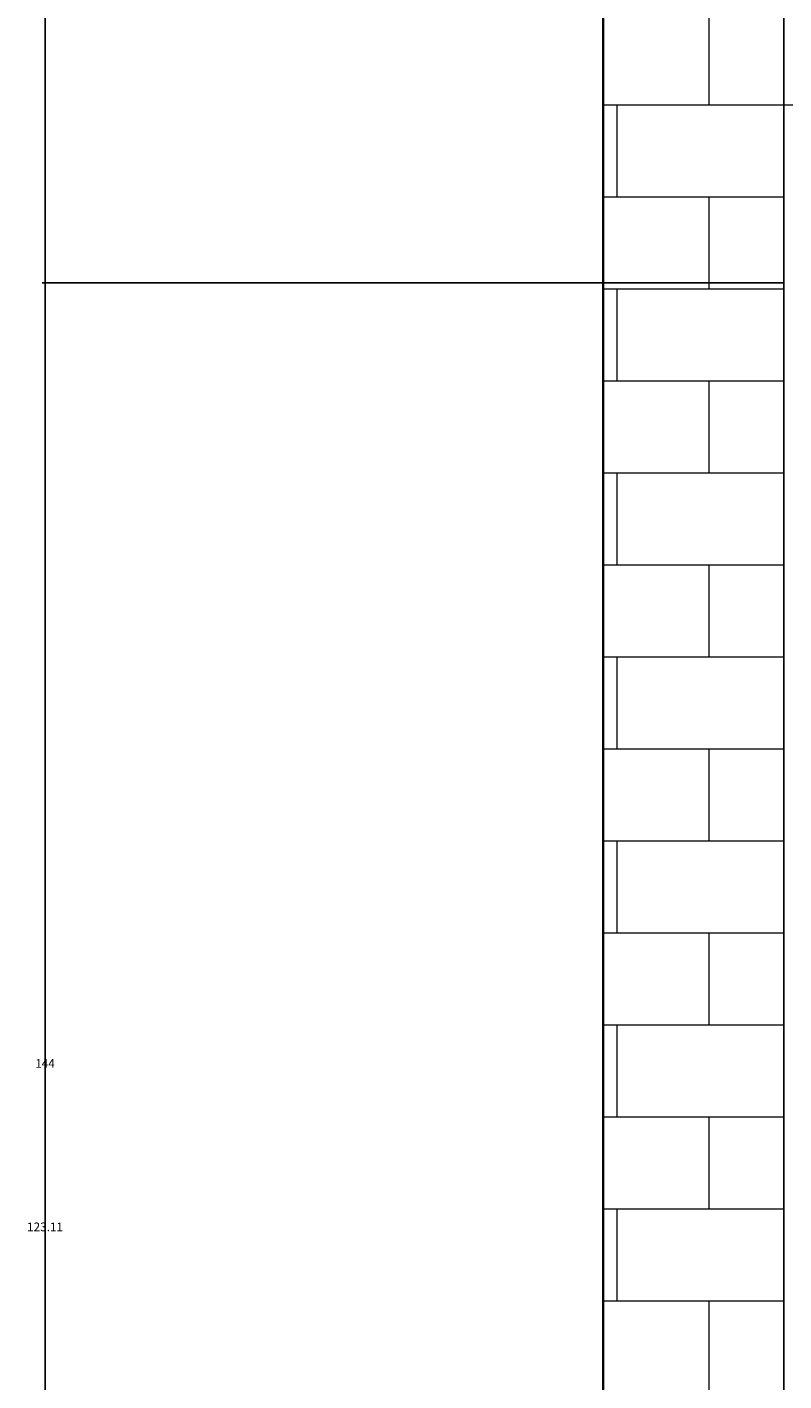
# Model space of a CAD drawing. Units: inches. Extents: x -26 to 776, y -22 to 650.
# Tile 3 of 62: x -26 to 23, y 67 to 155. Entities that reach past the tile are written whole.
import ezdxf

# ---------------------------------------------------------------- set-up
doc = ezdxf.new("R2010")
doc.units = ezdxf.units.IN
doc.header["$MEASUREMENT"] = 0
for name, color, linetype, lineweight in [('A-ANNO-DIMS', 2, 'Continuous', 18), ('A-WALL', 7, 'Continuous', 35), ('A-WALL-PATT', 8, 'Continuous', 13)]:
    doc.layers.add(name, color=color, linetype=linetype, lineweight=lineweight)
doc.styles.get("Standard").update_dxf_attribs({"font": 'arial.ttf'})
doc.dimstyles.get("Standard").update_dxf_attribs({"dimtxt": 0.5625, "dimasz": 0.18, "dimexe": 0.18, "dimexo": 0.0625, "dimgap": 0.09, "dimtad": 0, "dimtih": 1, "dimtoh": 1, "dimdec": 4, "dimzin": 0, "dimdsep": 46, "dimlunit": 4, "dimtxsty": 'Standard', "dimcen": 0.09, "dimadec": 0, "dimazin": 0, "dimtfac": 1, "dimtdec": 4, "dimtofl": 0, "dimtmove": 0, "dimatfit": 3, "dimfxl": 1, "dimtolj": 1, "dimtzin": 0, "dimarcsym": 0})

# ---------------------------------------------------------------- blocks, each defined once
blk = doc.blocks.new('*D14')
at = {"layer": 'A-ANNO-DIMS', "color": 0, "lineweight": -2, "transparency": 16777216}
for p, q in [((191.616, 613.271), (-25.478, 613.271)), ((-25.298, 613.091), (-25.298, 314.754)), ((-25.298, 15.662), (-25.298, 314)), ((11.045, 15.482), (-25.478, 15.482))]:
    blk.add_line(p, q, dxfattribs=at)
at = {"layer": 'A-ANNO-DIMS', "color": 0, "transparency": 16777216}
for points in [[(-25.328, 613.091), (-25.268, 613.091), (-25.298, 613.271)], [(-25.328, 15.662), (-25.268, 15.662), (-25.298, 15.482)]]:
    blk.add_solid(points, dxfattribs=at)
at = {"layer": 'Defpoints', "color": 0, "transparency": 16777216}
for p in [(-25.298, 613.271), (191.678, 613.271), (11.107, 15.482)]:
    blk.add_point(p, dxfattribs=at)
at = {"layer": 'A-ANNO-DIMS', "color": 0, "transparency": 16777216, "insert": (-25.298, 314.377), "char_height": 0.5625, "attachment_point": 5}
blk.add_mtext('\\A1;597.8', dxfattribs=at)
blk = doc.blocks.new('*D22')
at = {"layer": 'A-ANNO-DIMS', "color": 0, "lineweight": -2, "transparency": 16777216}
for p, q in [((22.889, 15.333), (22.889, 649.856)), ((217.953, 15.545), (217.953, 649.856)), ((23.069, 649.676), (119.19, 649.676)), ((217.773, 649.676), (121.652, 649.676))]:
    blk.add_line(p, q, dxfattribs=at)
at = {"layer": 'A-ANNO-DIMS', "color": 0, "transparency": 16777216}
for points in [[(23.069, 649.706), (23.069, 649.646), (22.889, 649.676)], [(217.773, 649.706), (217.773, 649.646), (217.953, 649.676)]]:
    blk.add_solid(points, dxfattribs=at)
at = {"layer": 'Defpoints', "color": 0, "transparency": 16777216}
for p in [(217.953, 649.676), (22.889, 15.27), (217.953, 15.482)]:
    blk.add_point(p, dxfattribs=at)
at = {"layer": 'A-ANNO-DIMS', "color": 0, "transparency": 16777216, "insert": (120.421, 649.676), "char_height": 0.5625, "attachment_point": 5}
blk.add_mtext('\\A1;195.06', dxfattribs=at)
blk = doc.blocks.new('*D23')
at = {"layer": 'A-ANNO-DIMS', "color": 0, "lineweight": -2, "transparency": 16777216}
for p, q in [((22.827, 138.384), (-25.478, 138.384)), ((-25.298, 138.204), (-25.298, 77.205)), ((-25.298, 15.45), (-25.298, 76.45)), ((22.827, 15.27), (-25.478, 15.27))]:
    blk.add_line(p, q, dxfattribs=at)
at = {"layer": 'A-ANNO-DIMS', "color": 0, "transparency": 16777216}
for points in [[(-25.328, 138.204), (-25.268, 138.204), (-25.298, 138.384)], [(-25.328, 15.45), (-25.268, 15.45), (-25.298, 15.27)]]:
    blk.add_solid(points, dxfattribs=at)
at = {"layer": 'Defpoints', "color": 0, "transparency": 16777216}
for p in [(-25.298, 138.384), (22.889, 138.384), (22.889, 15.27)]:
    blk.add_point(p, dxfattribs=at)
at = {"layer": 'A-ANNO-DIMS', "color": 0, "transparency": 16777216, "insert": (-25.298, 76.827), "char_height": 0.5625, "attachment_point": 5}
blk.add_mtext('\\A1;123.11', dxfattribs=at)
blk = doc.blocks.new('*D24')
at = {"layer": 'A-ANNO-DIMS', "color": 0, "lineweight": -2, "transparency": 16777216}
for p, q in [((11.107, 15.545), (11.107, 649.856)), ((22.889, 15.333), (22.889, 649.856)), ((11.287, 649.676), (15.77, 649.676)), ((22.709, 649.676), (18.226, 649.676))]:
    blk.add_line(p, q, dxfattribs=at)
at = {"layer": 'A-ANNO-DIMS', "color": 0, "transparency": 16777216}
for points in [[(11.287, 649.706), (11.287, 649.646), (11.107, 649.676)], [(22.709, 649.706), (22.709, 649.646), (22.889, 649.676)]]:
    blk.add_solid(points, dxfattribs=at)
at = {"layer": 'Defpoints', "color": 0, "transparency": 16777216}
for p in [(22.889, 649.676), (11.107, 15.482), (22.889, 15.27)]:
    blk.add_point(p, dxfattribs=at)
at = {"layer": 'A-ANNO-DIMS', "color": 0, "transparency": 16777216, "insert": (16.998, 649.676), "char_height": 0.5625, "attachment_point": 5}
blk.add_mtext('\\A1;11.782', dxfattribs=at)
blk = doc.blocks.new('*D37')
at = {"layer": 'A-ANNO-DIMS', "color": 0, "lineweight": -2, "transparency": 16777216}
for p, q in [((231.362, 159.482), (-25.478, 159.482)), ((-25.298, 159.302), (-25.298, 87.855)), ((-25.298, 15.662), (-25.298, 87.11)), ((217.89, 15.482), (-25.478, 15.482))]:
    blk.add_line(p, q, dxfattribs=at)
at = {"layer": 'A-ANNO-DIMS', "color": 0, "transparency": 16777216}
for points in [[(-25.328, 159.302), (-25.268, 159.302), (-25.298, 159.482)], [(-25.328, 15.662), (-25.268, 15.662), (-25.298, 15.482)]]:
    blk.add_solid(points, dxfattribs=at)
at = {"layer": 'Defpoints', "color": 0, "transparency": 16777216}
for p in [(-25.298, 159.482), (231.425, 159.482), (217.953, 15.482)]:
    blk.add_point(p, dxfattribs=at)
at = {"layer": 'A-ANNO-DIMS', "color": 0, "transparency": 16777216, "insert": (-25.298, 87.482), "char_height": 0.5625, "attachment_point": 5}
blk.add_mtext('\\A1;144', dxfattribs=at)

msp = doc.modelspace()

# ---------------------------------------------------------------- hatches: boundary and pattern name
at = {"layer": 'A-WALL-PATT'}
h = msp.add_hatch(dxfattribs=at)
h.set_pattern_fill('AR-B816', color=256, scale=0.75)
h.paths.add_polyline_path([(82.134, 209.6413), (11.1074, 209.6413), (11.1074, 159.4824), (82.134, 159.4824)])
h.paths.add_polyline_path([(231.4249, 209.6413), (209.091, 209.6413), (209.091, 159.4824), (214.1056, 159.4824), (214.1056, 199.3298), (231.4249, 199.3298)])
h.paths.add_polyline_path([(231.4249, 159.4824), (11.1074, 159.4824), (11.1074, 22.5014), (22.8891, 22.5014), (22.8891, 147.0781), (217.9529, 147.0781), (217.9529, 20.7937), (231.4249, 20.7937)])
h.paths.add_polyline_path([(285.0179, 152.3087), (280.6173, 144.8359), (280.6173, 26.4239), (240.1654, 26.4239), (240.1654, 144.8359), (231.4249, 159.4824), (231.4249, 20.7937), (285.0179, 20.7937)])

# ---------------------------------------------------------------- linework, layer by layer
at = {"layer": 'A-WALL'}
msp.add_line((11.1074, 15.4824), (11.1074, 159.4824), dxfattribs=at)

# ---------------------------------------------------------------- dimensions: what is measured, and where the dimension line sits
at = {"layer": 'A-ANNO-DIMS'}
for base, p1, p2, override, picture, middle in [((22.8891, 649.6763), (11.1074, 15.4824), (22.8891, 15.2701), {"dimdec": 3, "dimlfac": 1, "dimrnd": 0, "dimzin": 0, "dimdsep": 46, "dimlunit": 2}, '*D24', (16.9982, 649.6763)), ((217.9529, 649.6763), (22.8891, 15.2701), (217.9529, 15.4824), {"dimdec": 2, "dimlfac": 1, "dimrnd": 0, "dimzin": 0, "dimdsep": 46, "dimlunit": 2}, '*D22', (120.421, 649.6763))]:
    dim = msp.add_linear_dim(base=base, p1=p1, p2=p2, dimstyle='Standard', override=override, dxfattribs=at)
    dim.commit()
    dim.dimension.update_dxf_attribs({"geometry": picture, "text_midpoint": middle})
for base, p1, p2, override, picture, middle in [((-25.2976, 613.2713), (11.1074, 15.4824), (191.6782, 613.2713), {"dimdec": 1, "dimlfac": 1, "dimrnd": 0, "dimzin": 0, "dimdsep": 46, "dimlunit": 2}, '*D14', (-25.2976, 314.3769)), ((-25.2976, 159.4824), (217.9529, 15.4824), (231.4249, 159.4824), {"dimdec": 0, "dimlfac": 1, "dimrnd": 0, "dimzin": 0, "dimdsep": 46, "dimlunit": 2}, '*D37', (-25.2976, 87.4824)), ((-25.2976, 138.3844), (22.8891, 15.2701), (22.8891, 138.3844), {"dimdec": 2, "dimlfac": 1, "dimrnd": 0, "dimzin": 0, "dimdsep": 46, "dimlunit": 2}, '*D23', (-25.2976, 76.8273))]:
    dim = msp.add_linear_dim(base=base, p1=p1, p2=p2, angle=90, dimstyle='Standard', override=override, dxfattribs=at)
    dim.commit()
    dim.dimension.update_dxf_attribs({"geometry": picture, "text_midpoint": middle})

doc.saveas('drawing.dxf')
